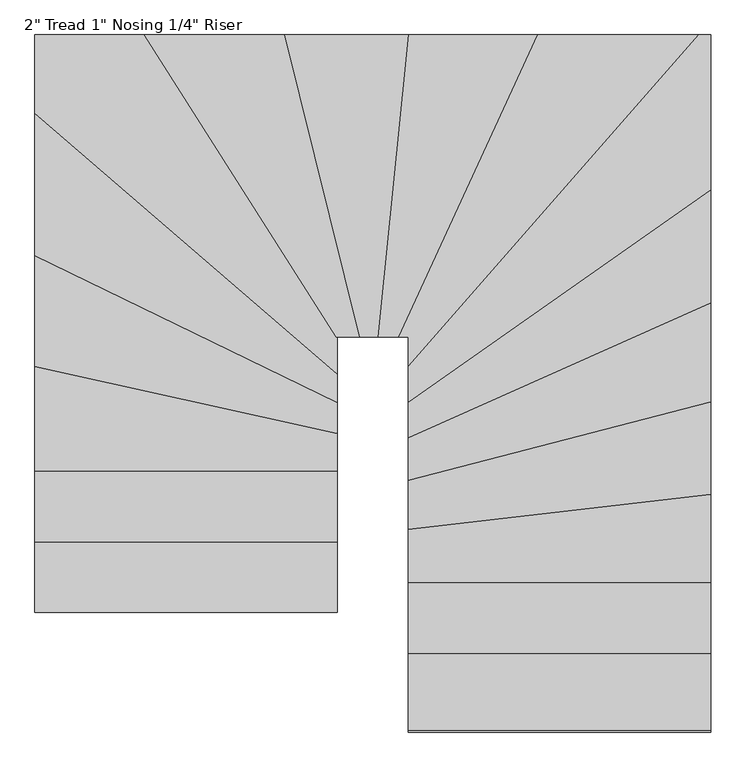
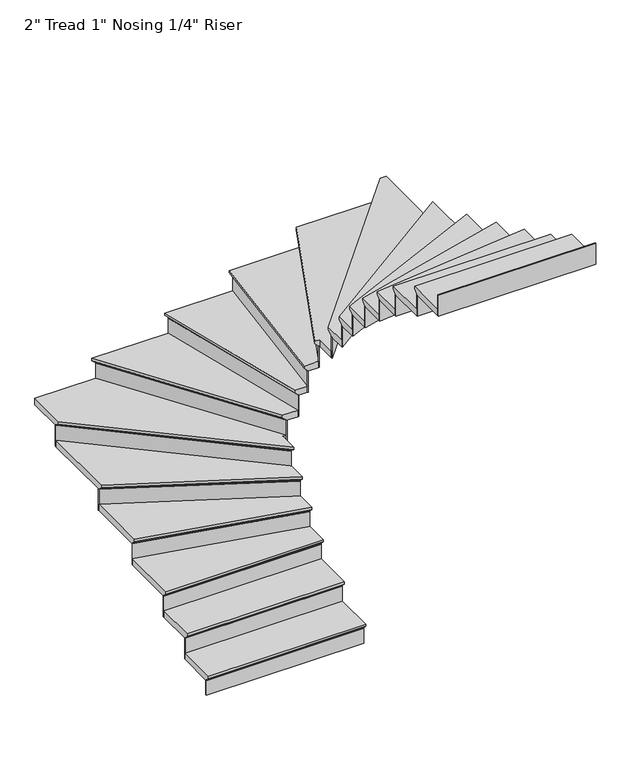
"""IFC4 building model written with IfcOpenShell, lengths in millimetres: stair flight geometry."""

from ifc_helpers import new_model, si_unit, origin, place, context, project, spatial, faceted_brep, source, transform, mapped, element, save


def stair_flight_8a5f7a69(model_context):
    return source(origin(), model_context, "Body", "Brep", [
        faceted_brep([(-1146.3860513, 5356.2607598, 150.2833333), (-1146.3860513, 5356.2607598, 169.3333333), (-2338.9053008, 5356.2607598, 169.3333333), (-2338.9053008, 5356.2607598, 150.2833333), (-1146.3860513, 5381.6607598, 124.8833333), (-2338.9053008, 5381.6607598, 124.8833333), (-1146.3860513, 5661.0607598, 169.3333333), (-2338.9053008, 5661.0607598, 169.3333333), (-2338.9053008, 5381.6607598, 118.5333333), (-2338.9053008, 5661.0607598, 118.5333333), (-1146.3860513, 5661.0607598, 118.5333333), (-1146.3860513, 5381.6607598, 118.5333333)], [[[0, 1, 2, 3]], [[4, 0, 3, 5]], [[2, 1, 6, 7]], [[8, 9, 10, 11]], [[2, 7, 9, 8, 5, 3]], [[8, 11, 4, 5]], [[6, 1, 0, 4, 11, 10]], [[7, 6, 10, 9]]]),
        faceted_brep([(-1146.3860513, 5381.6607598, 118.5333333), (-1146.3860513, 5381.6607598, 0.0), (-1146.3860513, 5388.0107598, 0.0), (-1146.3860513, 5388.0107598, 118.5333333), (-2338.9053008, 5381.6607598, 118.5333333), (-2338.9053008, 5388.0107598, 118.5333333), (-2338.9053008, 5388.0107598, 0.0), (-2338.9053008, 5381.6607598, 0.0)], [[[0, 1, 2, 3]], [[4, 5, 6, 7]], [[1, 0, 4, 7]], [[2, 1, 7, 6]], [[3, 2, 6, 5]], [[0, 3, 5, 4]]]),
        faceted_brep([(-1146.3860513, 5661.0607598, 287.8666667), (-1146.3860513, 5661.0607598, 118.5333333), (-1146.3860513, 5667.4107598, 118.5333333), (-1146.3860513, 5667.4107598, 287.8666667), (-2338.9053008, 5661.0607598, 287.8666667), (-2338.9053008, 5667.4107598, 287.8666667), (-2338.9053008, 5667.4107598, 118.5333333), (-2338.9053008, 5661.0607598, 118.5333333)], [[[0, 1, 2, 3]], [[4, 5, 6, 7]], [[1, 0, 4, 7]], [[2, 1, 7, 6]], [[3, 2, 6, 5]], [[0, 3, 5, 4]]]),
        faceted_brep([(-2338.9053008, 5635.6607598, 338.6666667), (-1146.3860513, 5635.6607598, 338.6666667), (-1146.3860513, 5940.4607598, 338.6666667), (-2338.9053008, 5940.4607598, 338.6666667), (-2338.9053008, 5661.0607598, 287.8666667), (-2338.9053008, 5940.4607598, 287.8666667), (-1146.3860513, 5940.4607598, 287.8666667), (-1146.3860513, 5661.0607598, 287.8666667), (-2338.9053008, 5661.0607598, 294.2166667), (-2338.9053008, 5635.6607598, 319.6166667), (-1146.3860513, 5661.0607598, 294.2166667), (-1146.3860513, 5635.6607598, 319.6166667)], [[[0, 1, 2, 3]], [[4, 5, 6, 7]], [[0, 3, 5, 4, 8, 9]], [[4, 7, 10, 8]], [[2, 1, 11, 10, 7, 6]], [[3, 2, 6, 5]], [[11, 1, 0, 9]], [[10, 11, 9, 8]]]),
        faceted_brep([(-1146.3860513, 5940.4607598, 457.2), (-1146.3860513, 5940.4607598, 287.8666667), (-1146.3860513, 5946.8107598, 287.8666667), (-1146.3860513, 5946.8107598, 457.2), (-2338.9053008, 5940.4607598, 457.2), (-2338.9053008, 5946.8107598, 457.2), (-2338.9053008, 5946.8107598, 287.8666667), (-2338.9053008, 5940.4607598, 287.8666667)], [[[0, 1, 2, 3]], [[4, 5, 6, 7]], [[1, 0, 4, 7]], [[2, 1, 7, 6]], [[3, 2, 6, 5]], [[0, 3, 5, 4]]]),
        faceted_brep([(-2338.9053008, 5915.0607598, 508.0), (-1146.3860513, 5915.0607598, 508.0), (-1146.3860513, 6088.5833614, 508.0), (-2338.9053008, 6352.3661013, 508.0), (-2338.9053008, 5940.4607598, 457.2), (-2338.9053008, 6352.3661013, 457.2), (-1146.3860513, 6088.5833614, 457.2), (-1146.3860513, 5940.4607598, 457.2), (-2338.9053008, 5940.4607598, 463.55), (-2338.9053008, 5915.0607598, 488.95), (-1146.3860513, 5940.4607598, 463.55), (-1146.3860513, 5915.0607598, 488.95)], [[[0, 1, 2, 3]], [[4, 5, 6, 7]], [[0, 3, 5, 4, 8, 9]], [[4, 7, 10, 8]], [[2, 1, 11, 10, 7, 6]], [[3, 2, 6, 5]], [[11, 1, 0, 9]], [[10, 11, 9, 8]]]),
        faceted_brep([(-1146.3860513, 6088.5833614, 626.5333333), (-1146.3860513, 6088.5833614, 457.2), (-1146.3860513, 6095.0868543, 457.2), (-1146.3860513, 6095.0868543, 626.5333333), (-2338.9053008, 6352.3661013, 626.5333333), (-2338.9053008, 6358.8695942, 626.5333333), (-2338.9053008, 6358.8695942, 457.2), (-2338.9053008, 6352.3661013, 457.2)], [[[0, 1, 2, 3]], [[4, 5, 6, 7]], [[1, 0, 4, 7]], [[2, 1, 7, 6]], [[3, 2, 6, 5]], [[0, 3, 5, 4]]]),
        faceted_brep([(-2338.9053008, 6326.3521298, 677.3333333), (-1146.3860513, 6062.5693899, 677.3333333), (-1146.3860513, 6212.87642, 677.3333333), (-2338.9053008, 6792.1477279, 677.3333333), (-2338.9053008, 6352.3661013, 626.5333333), (-2338.9053008, 6792.1477279, 626.5333333), (-1146.3860513, 6212.87642, 626.5333333), (-1146.3860513, 6088.5833614, 626.5333333), (-2338.9053008, 6352.3661013, 632.8833333), (-2338.9053008, 6326.3521298, 658.2833333), (-1146.3860513, 6088.5833614, 632.8833333), (-1146.3860513, 6062.5693899, 658.2833333)], [[[0, 1, 2, 3]], [[4, 5, 6, 7]], [[0, 3, 5, 4, 8, 9]], [[4, 7, 10, 8]], [[2, 1, 11, 10, 7, 6]], [[3, 2, 6, 5]], [[11, 1, 0, 9]], [[10, 11, 9, 8]]]),
        faceted_brep([(-1146.3860513, 6212.87642, 795.8666667), (-1146.3860513, 6212.87642, 626.5333333), (-1146.3860513, 6219.9359444, 626.5333333), (-1146.3860513, 6219.9359444, 795.8666667), (-2338.9053008, 6792.1477279, 795.8666667), (-2338.9053008, 6799.2072523, 795.8666667), (-2338.9053008, 6799.2072523, 626.5333333), (-2338.9053008, 6792.1477279, 626.5333333)], [[[0, 1, 2, 3]], [[4, 5, 6, 7]], [[1, 0, 4, 7]], [[2, 1, 7, 6]], [[3, 2, 6, 5]], [[0, 3, 5, 4]]]),
        faceted_brep([(-2338.9053008, 6763.9096305, 846.6666667), (-1146.3860513, 6184.6383225, 846.6666667), (-1146.3860513, 6330.6344837, 846.6666667), (-2338.9053008, 7358.8771228, 846.6666667), (-2338.9053008, 6792.1477279, 795.8666667), (-2338.9053008, 7358.8771228, 795.8666667), (-1146.3860513, 6330.6344837, 795.8666667), (-1146.3860513, 6212.87642, 795.8666667), (-2338.9053008, 6792.1477279, 802.2166667), (-2338.9053008, 6763.9096305, 827.6166667), (-1146.3860513, 6212.87642, 802.2166667), (-1146.3860513, 6184.6383225, 827.6166667)], [[[0, 1, 2, 3]], [[4, 5, 6, 7]], [[0, 3, 5, 4, 8, 9]], [[4, 7, 10, 8]], [[2, 1, 11, 10, 7, 6]], [[3, 2, 6, 5]], [[11, 1, 0, 9]], [[10, 11, 9, 8]]]),
        faceted_brep([(-1146.3860513, 6330.6344837, 965.2), (-1146.3860513, 6330.6344837, 795.8666667), (-1146.3860513, 6339.0190445, 795.8666667), (-1146.3860513, 6339.0190445, 965.2), (-2338.9053008, 7358.8771228, 965.2), (-2338.9053008, 7367.2616837, 965.2), (-2338.9053008, 7367.2616837, 795.8666667), (-2338.9053008, 7358.8771228, 795.8666667)], [[[0, 1, 2, 3]], [[4, 5, 6, 7]], [[1, 0, 4, 7]], [[2, 1, 7, 6]], [[3, 2, 6, 5]], [[0, 3, 5, 4]]]),
        faceted_brep([(-1877.8161732, 7634.4896548, 1016.0), (-2338.9053008, 7634.4896548, 1016.0), (-2338.9053008, 7325.3388796, 1016.0), (-1146.3860513, 6297.0962404, 1016.0), (-1146.3860513, 6441.9704052, 1016.0), (-1119.9677237, 6441.9704052, 1016.0), (-2338.9053008, 7634.4896548, 965.2), (-1877.8161732, 7634.4896548, 965.2), (-1119.9677237, 6441.9704052, 965.2), (-1146.3860513, 6441.9704052, 965.2), (-1146.3860513, 6330.6344837, 965.2), (-2338.9053008, 7358.8771228, 965.2), (-1146.3860513, 6330.6344837, 971.55), (-2338.9053008, 7358.8771228, 971.55), (-1146.3860513, 6297.0962404, 996.95), (-2338.9053008, 7325.3388796, 996.95)], [[[0, 1, 2, 3, 4, 5]], [[6, 7, 8, 9, 10, 11]], [[1, 0, 7, 6]], [[11, 10, 12, 13]], [[4, 3, 14, 12, 10, 9]], [[0, 5, 8, 7]], [[14, 3, 2, 15]], [[12, 14, 15, 13]], [[2, 1, 6, 11, 13, 15]], [[5, 4, 9, 8]]]),
        faceted_brep([(-1119.9677237, 6441.9704052, 1134.5333333), (-1119.9677237, 6441.9704052, 965.2), (-1112.443944, 6441.9704052, 965.2), (-1112.443944, 6441.9704052, 1134.5333333), (-1877.8161732, 7634.4896548, 1134.5333333), (-1870.2923935, 7634.4896548, 1134.5333333), (-1870.2923935, 7634.4896548, 965.2), (-1877.8161732, 7634.4896548, 965.2)], [[[0, 1, 2, 3]], [[4, 5, 6, 7]], [[1, 0, 4, 7]], [[2, 1, 7, 6]], [[3, 2, 6, 5]], [[0, 3, 5, 4]]]),
        faceted_brep([(-1907.911292, 7634.4896548, 1185.3333333), (-1150.0628425, 6441.9704052, 1185.3333333), (-1031.6046528, 6441.9704052, 1185.3333333), (-1327.3357944, 7634.4896548, 1185.3333333), (-1877.8161732, 7634.4896548, 1134.5333333), (-1327.3357944, 7634.4896548, 1134.5333333), (-1031.6046528, 6441.9704052, 1134.5333333), (-1119.9677237, 6441.9704052, 1134.5333333), (-1877.8161732, 7634.4896548, 1140.8833333), (-1907.911292, 7634.4896548, 1166.2833333), (-1119.9677237, 6441.9704052, 1140.8833333), (-1150.0628425, 6441.9704052, 1166.2833333)], [[[0, 1, 2, 3]], [[4, 5, 6, 7]], [[0, 3, 5, 4, 8, 9]], [[4, 7, 10, 8]], [[2, 1, 11, 10, 7, 6]], [[3, 2, 6, 5]], [[11, 1, 0, 9]], [[10, 11, 9, 8]]]),
        faceted_brep([(-1031.6046528, 6441.9704052, 1303.8666667), (-1031.6046528, 6441.9704052, 1134.5333333), (-1025.0623087, 6441.9704052, 1134.5333333), (-1025.0623087, 6441.9704052, 1303.8666667), (-1327.3357944, 7634.4896548, 1303.8666667), (-1320.7934503, 7634.4896548, 1303.8666667), (-1320.7934503, 7634.4896548, 1134.5333333), (-1327.3357944, 7634.4896548, 1134.5333333)], [[[0, 1, 2, 3]], [[4, 5, 6, 7]], [[1, 0, 4, 7]], [[2, 1, 7, 6]], [[3, 2, 6, 5]], [[0, 3, 5, 4]]]),
        faceted_brep([(-1353.5051708, 7634.4896548, 1354.6666667), (-1057.7740293, 6441.9704052, 1354.6666667), (-960.2447552, 6441.9704052, 1354.6666667), (-839.7768987, 7634.4896548, 1354.6666667), (-1327.3357944, 7634.4896548, 1303.8666667), (-839.7768987, 7634.4896548, 1303.8666667), (-960.2447552, 6441.9704052, 1303.8666667), (-1031.6046528, 6441.9704052, 1303.8666667), (-1327.3357944, 7634.4896548, 1310.2166667), (-1353.5051708, 7634.4896548, 1335.6166667), (-1031.6046528, 6441.9704052, 1310.2166667), (-1057.7740293, 6441.9704052, 1335.6166667)], [[[0, 1, 2, 3]], [[4, 5, 6, 7]], [[0, 3, 5, 4, 8, 9]], [[4, 7, 10, 8]], [[3, 2, 6, 5]], [[11, 1, 0, 9]], [[10, 11, 9, 8]], [[2, 1, 11, 10, 7, 6]]]),
        faceted_brep([(-960.2447552, 6441.9704052, 1473.2), (-960.2447552, 6441.9704052, 1303.8666667), (-953.8624366, 6441.9704052, 1303.8666667), (-953.8624366, 6441.9704052, 1473.2), (-839.7768987, 7634.4896548, 1473.2), (-833.3945802, 7634.4896548, 1473.2), (-833.3945802, 7634.4896548, 1303.8666667), (-839.7768987, 7634.4896548, 1303.8666667)], [[[0, 1, 2, 3]], [[4, 5, 6, 7]], [[1, 0, 4, 7]], [[2, 1, 7, 6]], [[3, 2, 6, 5]], [[0, 3, 5, 4]]]),
        faceted_brep([(-865.3061728, 7634.4896548, 1524.0), (-985.7740293, 6441.9704052, 1524.0), (-876.4170654, 6441.9704052, 1524.0), (-328.1794285, 7634.4896548, 1524.0), (-839.7768987, 7634.4896548, 1473.2), (-328.1794285, 7634.4896548, 1473.2), (-876.4170654, 6441.9704052, 1473.2), (-960.2447552, 6441.9704052, 1473.2), (-839.7768987, 7634.4896548, 1479.55), (-865.3061728, 7634.4896548, 1504.95), (-960.2447552, 6441.9704052, 1479.55), (-985.7740293, 6441.9704052, 1504.95)], [[[0, 1, 2, 3]], [[4, 5, 6, 7]], [[0, 3, 5, 4, 8, 9]], [[4, 7, 10, 8]], [[2, 1, 11, 10, 7, 6]], [[3, 2, 6, 5]], [[11, 1, 0, 9]], [[10, 11, 9, 8]]]),
        faceted_brep([(-876.4170654, 6441.9704052, 1642.5333333), (-876.4170654, 6441.9704052, 1473.2), (-869.4281633, 6441.9704052, 1473.2), (-869.4281633, 6441.9704052, 1642.5333333), (-328.1794285, 7634.4896548, 1642.5333333), (-321.1905265, 7634.4896548, 1642.5333333), (-321.1905265, 7634.4896548, 1473.2), (-328.1794285, 7634.4896548, 1473.2)], [[[0, 1, 2, 3]], [[4, 5, 6, 7]], [[1, 0, 4, 7]], [[2, 1, 7, 6]], [[3, 2, 6, 5]], [[0, 3, 5, 4]]]),
        faceted_brep([(-356.1350366, 7634.4896548, 1693.3333333), (-904.3726735, 6441.9704052, 1693.3333333), (-866.9860513, 6441.9704052, 1693.3333333), (-866.9860513, 6288.8084089, 1693.3333333), (312.829045, 7634.4896548, 1693.3333333), (-328.1794285, 7634.4896548, 1642.5333333), (312.829045, 7634.4896548, 1642.5333333), (-866.9860513, 6288.8084089, 1642.5333333), (-866.9860513, 6441.9704052, 1642.5333333), (-876.4170654, 6441.9704052, 1642.5333333), (-328.1794285, 7634.4896548, 1648.8833333), (-356.1350366, 7634.4896548, 1674.2833333), (-876.4170654, 6441.9704052, 1648.8833333), (-904.3726735, 6441.9704052, 1674.2833333)], [[[0, 1, 2, 3, 4]], [[5, 6, 7, 8, 9]], [[0, 4, 6, 5, 10, 11]], [[5, 9, 12, 10]], [[2, 1, 13, 12, 9, 8]], [[3, 2, 8, 7]], [[4, 3, 7, 6]], [[13, 1, 0, 11]], [[12, 13, 11, 10]]]),
        faceted_brep([(-866.9860513, 6288.8084089, 1811.8666667), (-866.9860513, 6288.8084089, 1642.5333333), (-866.9860513, 6279.1761942, 1642.5333333), (-866.9860513, 6279.1761942, 1811.8666667), (312.829045, 7634.4896548, 1811.8666667), (321.274011, 7634.4896548, 1811.8666667), (321.274011, 7634.4896548, 1642.5333333), (312.829045, 7634.4896548, 1642.5333333)], [[[0, 1, 2, 3]], [[4, 5, 6, 7]], [[1, 0, 4, 7]], [[2, 1, 7, 6]], [[3, 2, 6, 5]], [[0, 3, 5, 4]]]),
        faceted_brep([(325.5331983, 6990.2330522, 1862.6666667), (325.5331983, 7634.4896548, 1862.6666667), (279.049181, 7634.4896548, 1862.6666667), (-866.9860513, 6327.3372678, 1862.6666667), (-866.9860513, 6153.935953, 1862.6666667), (325.5331983, 7634.4896548, 1811.8666667), (325.5331983, 6990.2330522, 1811.8666667), (-866.9860513, 6153.935953, 1811.8666667), (-866.9860513, 6288.8084089, 1811.8666667), (312.829045, 7634.4896548, 1811.8666667), (312.829045, 7634.4896548, 1818.2166667), (279.049181, 7634.4896548, 1843.6166667), (-866.9860513, 6288.8084089, 1818.2166667), (-866.9860513, 6327.3372678, 1843.6166667)], [[[0, 1, 2, 3, 4]], [[5, 6, 7, 8, 9]], [[1, 0, 6, 5]], [[2, 1, 5, 9, 10, 11]], [[9, 8, 12, 10]], [[4, 3, 13, 12, 8, 7]], [[0, 4, 7, 6]], [[13, 3, 2, 11]], [[12, 13, 11, 10]]]),
        faceted_brep([(-866.9860513, 6153.935953, 1981.2), (-866.9860513, 6153.935953, 1811.8666667), (-866.9860513, 6146.1801042, 1811.8666667), (-866.9860513, 6146.1801042, 1981.2), (325.5331983, 6990.2330522, 1981.2), (325.5331983, 6982.4772034, 1981.2), (325.5331983, 6982.4772034, 1811.8666667), (325.5331983, 6990.2330522, 1811.8666667)], [[[0, 1, 2, 3]], [[4, 5, 6, 7]], [[1, 0, 4, 7]], [[2, 1, 7, 6]], [[3, 2, 6, 5]], [[0, 3, 5, 4]]]),
        faceted_brep([(325.5331983, 7021.2564474, 2032.0), (-866.9860513, 6184.9593481, 2032.0), (-866.9860513, 6017.2382603, 2032.0), (325.5331983, 6549.6069274, 2032.0), (325.5331983, 6990.2330522, 1981.2), (325.5331983, 6549.6069274, 1981.2), (-866.9860513, 6017.2382603, 1981.2), (-866.9860513, 6153.935953, 1981.2), (325.5331983, 6990.2330522, 1987.55), (325.5331983, 7021.2564474, 2012.95), (-866.9860513, 6153.935953, 1987.55), (-866.9860513, 6184.9593481, 2012.95)], [[[0, 1, 2, 3]], [[4, 5, 6, 7]], [[0, 3, 5, 4, 8, 9]], [[4, 7, 10, 8]], [[2, 1, 11, 10, 7, 6]], [[3, 2, 6, 5]], [[11, 1, 0, 9]], [[10, 11, 9, 8]]]),
        faceted_brep([(-866.9860513, 6017.2382603, 2150.5333333), (-866.9860513, 6017.2382603, 1981.2), (-866.9860513, 6010.2842304, 1981.2), (-866.9860513, 6010.2842304, 2150.5333333), (325.5331983, 6549.6069274, 2150.5333333), (325.5331983, 6542.6528975, 2150.5333333), (325.5331983, 6542.6528975, 1981.2), (325.5331983, 6549.6069274, 1981.2)], [[[0, 1, 2, 3]], [[4, 5, 6, 7]], [[1, 0, 4, 7]], [[2, 1, 7, 6]], [[3, 2, 6, 5]], [[0, 3, 5, 4]]]),
        faceted_brep([(325.5331983, 6577.4230469, 2201.3333333), (-866.9860513, 6045.0543798, 2201.3333333), (-866.9860513, 5850.1664403, 2201.3333333), (325.5331983, 6161.0135225, 2201.3333333), (325.5331983, 6549.6069274, 2150.5333333), (325.5331983, 6161.0135225, 2150.5333333), (-866.9860513, 5850.1664403, 2150.5333333), (-866.9860513, 6017.2382603, 2150.5333333), (325.5331983, 6549.6069274, 2156.8833333), (325.5331983, 6577.4230469, 2182.2833333), (-866.9860513, 6017.2382603, 2156.8833333), (-866.9860513, 6045.0543798, 2182.2833333)], [[[0, 1, 2, 3]], [[4, 5, 6, 7]], [[0, 3, 5, 4, 8, 9]], [[4, 7, 10, 8]], [[2, 1, 11, 10, 7, 6]], [[3, 2, 6, 5]], [[11, 1, 0, 9]], [[10, 11, 9, 8]]]),
        faceted_brep([(-866.9860513, 5850.1664403, 2319.8666667), (-866.9860513, 5850.1664403, 2150.5333333), (-866.9860513, 5843.6042573, 2150.5333333), (-866.9860513, 5843.6042573, 2319.8666667), (325.5331983, 6161.0135225, 2319.8666667), (325.5331983, 6154.4513395, 2319.8666667), (325.5331983, 6154.4513395, 2150.5333333), (325.5331983, 6161.0135225, 2150.5333333)], [[[0, 1, 2, 3]], [[4, 5, 6, 7]], [[1, 0, 4, 7]], [[2, 1, 7, 6]], [[3, 2, 6, 5]], [[0, 3, 5, 4]]]),
        faceted_brep([(325.5331983, 6187.2622544, 2370.6666667), (-866.9860513, 5876.4151722, 2370.6666667), (-866.9860513, 5657.7397324, 2370.6666667), (325.5331983, 5795.9974198, 2370.6666667), (325.5331983, 6161.0135225, 2319.8666667), (325.5331983, 5795.9974198, 2319.8666667), (-866.9860513, 5657.7397324, 2319.8666667), (-866.9860513, 5850.1664403, 2319.8666667), (325.5331983, 6161.0135225, 2326.2166667), (325.5331983, 6187.2622544, 2351.6166667), (-866.9860513, 5850.1664403, 2326.2166667), (-866.9860513, 5876.4151722, 2351.6166667)], [[[0, 1, 2, 3]], [[4, 5, 6, 7]], [[0, 3, 5, 4, 8, 9]], [[4, 7, 10, 8]], [[2, 1, 11, 10, 7, 6]], [[3, 2, 6, 5]], [[11, 1, 0, 9]], [[10, 11, 9, 8]]]),
        faceted_brep([(-866.9860513, 5657.7397324, 2489.2), (-866.9860513, 5657.7397324, 2319.8666667), (-866.9860513, 5651.3471981, 2319.8666667), (-866.9860513, 5651.3471981, 2489.2), (325.5331983, 5795.9974198, 2489.2), (325.5331983, 5789.6048854, 2489.2), (325.5331983, 5789.6048854, 2319.8666667), (325.5331983, 5795.9974198, 2319.8666667)], [[[0, 1, 2, 3]], [[4, 5, 6, 7]], [[1, 0, 4, 7]], [[2, 1, 7, 6]], [[3, 2, 6, 5]], [[0, 3, 5, 4]]]),
        faceted_brep([(325.5331983, 5821.567557, 2540.0), (-866.9860513, 5683.3098697, 2540.0), (-866.9860513, 5447.6387133, 2540.0), (325.5331983, 5447.6387133, 2540.0), (325.5331983, 5795.9974198, 2489.2), (325.5331983, 5447.6387133, 2489.2), (-866.9860513, 5447.6387133, 2489.2), (-866.9860513, 5657.7397324, 2489.2), (325.5331983, 5795.9974198, 2495.55), (325.5331983, 5821.567557, 2520.95), (-866.9860513, 5657.7397324, 2495.55), (-866.9860513, 5683.3098697, 2520.95)], [[[0, 1, 2, 3]], [[4, 5, 6, 7]], [[0, 3, 5, 4, 8, 9]], [[4, 7, 10, 8]], [[2, 1, 11, 10, 7, 6]], [[3, 2, 6, 5]], [[11, 1, 0, 9]], [[10, 11, 9, 8]]]),
        faceted_brep([(-866.9860513, 5447.6387133, 2658.5333333), (-866.9860513, 5447.6387133, 2489.2), (-866.9860513, 5441.2887133, 2489.2), (-866.9860513, 5441.2887133, 2658.5333333), (325.5331983, 5447.6387133, 2658.5333333), (325.5331983, 5441.2887133, 2658.5333333), (325.5331983, 5441.2887133, 2489.2), (325.5331983, 5447.6387133, 2489.2)], [[[0, 1, 2, 3]], [[4, 5, 6, 7]], [[1, 0, 4, 7]], [[2, 1, 7, 6]], [[3, 2, 6, 5]], [[0, 3, 5, 4]]]),
        faceted_brep([(325.5331983, 5473.0387133, 2709.3333333), (-866.9860513, 5473.0387133, 2709.3333333), (-866.9860513, 5168.2387133, 2709.3333333), (325.5331983, 5168.2387133, 2709.3333333), (325.5331983, 5447.6387133, 2658.5333333), (325.5331983, 5168.2387133, 2658.5333333), (-866.9860513, 5168.2387133, 2658.5333333), (-866.9860513, 5447.6387133, 2658.5333333), (325.5331983, 5447.6387133, 2664.8833333), (325.5331983, 5473.0387133, 2690.2833333), (-866.9860513, 5447.6387133, 2664.8833333), (-866.9860513, 5473.0387133, 2690.2833333)], [[[0, 1, 2, 3]], [[4, 5, 6, 7]], [[0, 3, 5, 4, 8, 9]], [[4, 7, 10, 8]], [[2, 1, 11, 10, 7, 6]], [[3, 2, 6, 5]], [[11, 1, 0, 9]], [[10, 11, 9, 8]]]),
        faceted_brep([(-866.9860513, 5168.2387133, 2827.8666667), (-866.9860513, 5168.2387133, 2658.5333333), (-866.9860513, 5161.8887133, 2658.5333333), (-866.9860513, 5161.8887133, 2827.8666667), (325.5331983, 5168.2387133, 2827.8666667), (325.5331983, 5161.8887133, 2827.8666667), (325.5331983, 5161.8887133, 2658.5333333), (325.5331983, 5168.2387133, 2658.5333333)], [[[0, 1, 2, 3]], [[4, 5, 6, 7]], [[1, 0, 4, 7]], [[2, 1, 7, 6]], [[3, 2, 6, 5]], [[0, 3, 5, 4]]]),
        faceted_brep([(-866.9860513, 4888.8387133, 2997.2), (-866.9860513, 4888.8387133, 2827.8666667), (-866.9860513, 4882.4887133, 2827.8666667), (-866.9860513, 4882.4887133, 2997.2), (325.5331983, 4888.8387133, 2997.2), (325.5331983, 4882.4887133, 2997.2), (325.5331983, 4882.4887133, 2827.8666667), (325.5331983, 4888.8387133, 2827.8666667)], [[[0, 1, 2, 3]], [[4, 5, 6, 7]], [[1, 0, 4, 7]], [[2, 1, 7, 6]], [[3, 2, 6, 5]], [[0, 3, 5, 4]]]),
        faceted_brep([(325.5331983, 5193.6387133, 2878.6666667), (-866.9860513, 5193.6387133, 2878.6666667), (-866.9860513, 4888.8387133, 2878.6666667), (325.5331983, 4888.8387133, 2878.6666667), (325.5331983, 5168.2387133, 2827.8666667), (325.5331983, 4888.8387133, 2827.8666667), (-866.9860513, 4888.8387133, 2827.8666667), (-866.9860513, 5168.2387133, 2827.8666667), (325.5331983, 5168.2387133, 2834.2166667), (325.5331983, 5193.6387133, 2859.6166667), (-866.9860513, 5168.2387133, 2834.2166667), (-866.9860513, 5193.6387133, 2859.6166667)], [[[0, 1, 2, 3]], [[4, 5, 6, 7]], [[0, 3, 5, 4, 8, 9]], [[4, 7, 10, 8]], [[2, 1, 11, 10, 7, 6]], [[3, 2, 6, 5]], [[11, 1, 0, 9]], [[10, 11, 9, 8]]]),
    ])


if __name__ == "__main__":
    model = new_model("IFC4")
    model_context = context("Model", 3, world=origin())
    ifc_project = project(units=[si_unit("LENGTHUNIT", "METRE", prefix="MILLI")], contexts=[model_context])
    site = spatial("IfcSite", under=ifc_project)
    building = spatial("IfcBuilding", under=site)
    placement = place(None, origin())
    stair_flight_shape = stair_flight_8a5f7a69(model_context)
    element("IfcStairFlight", 1, ObjectType="2\" Tread 1\" Nosing 1/4\" Riser", at=placement, inside=building, context=model_context, shape_type="MappedRepresentation", body=[
        mapped(stair_flight_shape, transform((0.0, 0.0, 0.0), x_axis=(1.0, 0.0, 0.0), y_axis=(0.0, 1.0, 0.0), z_axis=(0.0, 0.0, 1.0))),
    ])
    save(model, "model.ifc")
